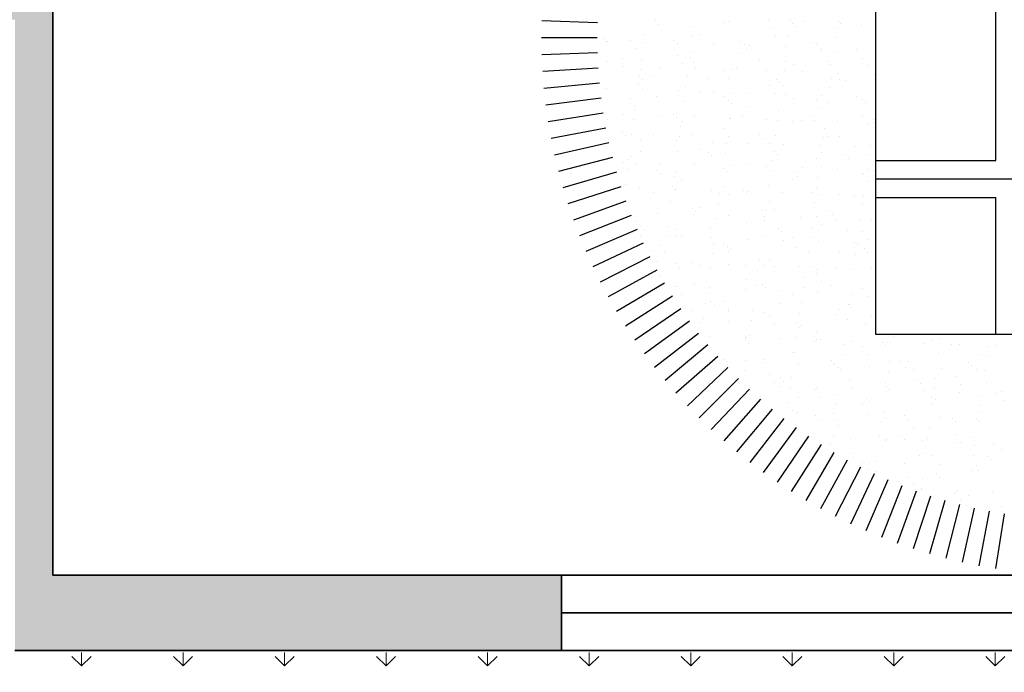
# Model space of a CAD drawing. Units: inches. Extents: x 1566 to 2546, y 1087 to 2705.
# Tile 3 of 27: x 1820 to 1925, y 1201 to 1270. Entities that reach past the tile are written whole.
import ezdxf

# ---------------------------------------------------------------- set-up
doc = ezdxf.new("R2010")
doc.units = ezdxf.units.IN
for name, color, linetype, lineweight in [('A-FLOR-PATT', 3, 'Continuous', 13), ('A-FURN', 8, 'Continuous', 18), ('A-WALL', 7, 'Continuous', 35), ('A-WALL-PATT', 8, 'Continuous', 13)]:
    doc.layers.add(name, color=color, linetype=linetype, lineweight=lineweight)
for name, color, linetype in [('A-FRN', 11, 'Continuous'), ('A-HT', 15, 'Continuous'), ('L-HT', 1, 'Continuous')]:
    doc.layers.add(name, color=color, linetype=linetype)

# ---------------------------------------------------------------- blocks, each defined once
blk = doc.blocks.new('*X21')
at = {"color": 0}
for p, q in [((2.0018, 2.8313), (2.0018, 2.8313)), ((2.0087, 2.8252), (2.0087, 2.8252)), ((2.011, 2.8229), (2.011, 2.8229)), ((2.0652, 2.8233), (2.0652, 2.8233)), ((2.1366, 2.8246), (2.1366, 2.8246)), ((2.2048, 2.8269), (2.2048, 2.8269)), ((2.2209, 2.8236), (2.2209, 2.8236)), ((2.0545, 2.783), (2.0545, 2.783)), ((2.0763, 2.7783), (2.0763, 2.7783)), ((2.2072, 2.78), (2.2072, 2.78)), ((2.2546, 2.7813), (2.2546, 2.7813)), ((2.2638, 2.7728), (2.2638, 2.7728)), ((2.32, 2.7605), (2.32, 2.7605)), ((2.3282, 2.7662), (2.3282, 2.7662)), ((2.3351, 2.7793), (2.3351, 2.7793)), ((2.3542, 2.7696), (2.3542, 2.7696)), ((2.3949, 2.775), (2.3949, 2.775)), ((2.0085, 2.7599), (2.0085, 2.7599)), ((2.0296, 2.7465), (2.0296, 2.7465)), ((2.0851, 2.7342), (2.0851, 2.7342)), ((2.1043, 2.7374), (2.1043, 2.7374)), ((2.1257, 2.7395), (2.1257, 2.7395)), ((2.1643, 2.7602), (2.1643, 2.7602)), ((2.1853, 2.7467), (2.1853, 2.7467)), ((2.1936, 2.7485), (2.1936, 2.7485)), ((2.2196, 2.7519), (2.2196, 2.7519)), ((2.2603, 2.7573), (2.2603, 2.7573)), ((2.341, 2.747), (2.341, 2.747)), ((2.4057, 2.7348), (2.4057, 2.7348)), ((2.4967, 2.7473), (2.4967, 2.7473)), ((2.5336, 2.7341), (2.5336, 2.7341)), ((1.9911, 2.7218), (1.9911, 2.7218)), ((2.0118, 2.7288), (2.0118, 2.7288)), ((2.059, 2.7308), (2.059, 2.7308)), ((2.1135, 2.729), (2.1135, 2.729)), ((2.1397, 2.7282), (2.1397, 2.7282)), ((2.2748, 2.7331), (2.2748, 2.7331)), ((2.3073, 2.733), (2.3073, 2.733)), ((2.5074, 2.7313), (2.5074, 2.7313)), ((2.5166, 2.7228), (2.5166, 2.7228)), ((1.954, 2.6935), (1.954, 2.6935)), ((1.9632, 2.6851), (1.9632, 2.6851)), ((2.0794, 2.682), (2.0794, 2.682)), ((2.1055, 2.6981), (2.1055, 2.6981)), ((2.157, 2.6891), (2.157, 2.6891)), ((2.2103, 2.6836), (2.2103, 2.6836)), ((2.2612, 2.6984), (2.2612, 2.6984)), ((2.3382, 2.683), (2.3382, 2.683)), ((2.3571, 2.6874), (2.3571, 2.6874)), ((2.4169, 2.6987), (2.4169, 2.6987)), ((2.4733, 2.6879), (2.4733, 2.6879)), ((2.5601, 2.683), (2.5601, 2.683)), ((2.5727, 2.6989), (2.5727, 2.6989)), ((2.6042, 2.6895), (2.6042, 2.6895)), ((2.3663, 2.6789), (2.3663, 2.6789)), ((2.5089, 2.6605), (2.5089, 2.6605)), ((2.5349, 2.664), (2.5349, 2.664)), ((2.5756, 2.6693), (2.5756, 2.6693)), ((2.6435, 2.6783), (2.6435, 2.6783)), ((2.0067, 2.6452), (2.0067, 2.6452)), ((2.015, 2.6325), (2.015, 2.6325)), ((2.0489, 2.6347), (2.0489, 2.6347)), ((2.1429, 2.6319), (2.1429, 2.6319)), ((2.2046, 2.635), (2.2046, 2.635)), ((2.2068, 2.6435), (2.2068, 2.6435)), ((2.216, 2.635), (2.216, 2.635)), ((2.2657, 2.6285), (2.2657, 2.6285)), ((2.2779, 2.6367), (2.2779, 2.6367)), ((2.3064, 2.6339), (2.3064, 2.6339)), ((2.3603, 2.6352), (2.3603, 2.6352)), ((2.3743, 2.6428), (2.3743, 2.6428)), ((2.4003, 2.6462), (2.4003, 2.6462)), ((2.4088, 2.6384), (2.4088, 2.6384)), ((2.4098, 2.6391), (2.4098, 2.6391)), ((2.441, 2.6516), (2.441, 2.6516)), ((2.516, 2.6355), (2.516, 2.6355)), ((2.5367, 2.6378), (2.5367, 2.6378)), ((2.6099, 2.6374), (2.6099, 2.6374)), ((2.6191, 2.6289), (2.6191, 2.6289)), ((2.6718, 2.6427), (2.6718, 2.6427)), ((2.6718, 2.6358), (2.6718, 2.6358)), ((2.07, 2.6213), (2.07, 2.6213)), ((2.1051, 2.6074), (2.1051, 2.6074)), ((2.1312, 2.6108), (2.1312, 2.6108)), ((2.1718, 2.6162), (2.1718, 2.6162)), ((2.2257, 2.6215), (2.2257, 2.6215)), ((2.2397, 2.6251), (2.2397, 2.6251)), ((2.3814, 2.6218), (2.3814, 2.6218)), ((2.5371, 2.6221), (2.5371, 2.6221)), ((2.6928, 2.6224), (2.6928, 2.6224)), ((1.9705, 2.5897), (1.9705, 2.5897)), ((1.9966, 2.5931), (1.9966, 2.5931)), ((2.0372, 2.5984), (2.0372, 2.5984)), ((2.0565, 2.5996), (2.0565, 2.5996)), ((2.0657, 2.5912), (2.0657, 2.5912)), ((2.0826, 2.5856), (2.0826, 2.5856)), ((2.2135, 2.5873), (2.2135, 2.5873)), ((2.2595, 2.5952), (2.2595, 2.5952)), ((2.3414, 2.5867), (2.3414, 2.5867)), ((2.4595, 2.5935), (2.4595, 2.5935)), ((2.4688, 2.585), (2.4688, 2.585)), ((2.4764, 2.5915), (2.4764, 2.5915)), ((2.6073, 2.5932), (2.6073, 2.5932)), ((2.6626, 2.589), (2.6626, 2.589)), ((2.7352, 2.5926), (2.7352, 2.5926)), ((1.9902, 2.5726), (1.9902, 2.5726)), ((2.1092, 2.5513), (2.1092, 2.5513)), ((2.1459, 2.5729), (2.1459, 2.5729)), ((2.3016, 2.5732), (2.3016, 2.5732)), ((2.3092, 2.5496), (2.3092, 2.5496)), ((2.4573, 2.5735), (2.4573, 2.5735)), ((2.613, 2.5737), (2.613, 2.5737)), ((2.6896, 2.5549), (2.6896, 2.5549)), ((2.7156, 2.5583), (2.7156, 2.5583)), ((2.7563, 2.5636), (2.7563, 2.5636)), ((2.7687, 2.574), (2.7687, 2.574)), ((2.0181, 2.5361), (2.0181, 2.5361)), ((2.146, 2.5355), (2.146, 2.5355)), ((2.2811, 2.5404), (2.2811, 2.5404)), ((2.3185, 2.5411), (2.3185, 2.5411)), ((2.412, 2.5421), (2.412, 2.5421)), ((2.4464, 2.5229), (2.4464, 2.5229)), ((2.4871, 2.5282), (2.4871, 2.5282)), ((2.5123, 2.5452), (2.5123, 2.5452)), ((2.5399, 2.5415), (2.5399, 2.5415)), ((2.555, 2.5371), (2.555, 2.5371)), ((2.581, 2.5406), (2.581, 2.5406)), ((2.6217, 2.5459), (2.6217, 2.5459)), ((2.6749, 2.5463), (2.6749, 2.5463)), ((2.7123, 2.5434), (2.7123, 2.5434)), ((2.7216, 2.535), (2.7216, 2.535)), ((2.8058, 2.548), (2.8058, 2.548)), ((1.9547, 2.4958), (1.9547, 2.4958)), ((1.9589, 2.5074), (1.9589, 2.5074)), ((2.0893, 2.5095), (2.0893, 2.5095)), ((2.1104, 2.496), (2.1104, 2.496)), ((2.1589, 2.5057), (2.1589, 2.5057)), ((2.1682, 2.4973), (2.1682, 2.4973)), ((2.245, 2.5098), (2.245, 2.5098)), ((2.2661, 2.4963), (2.2661, 2.4963)), ((2.2858, 2.5017), (2.2858, 2.5017)), ((2.3118, 2.5051), (2.3118, 2.5051)), ((2.3525, 2.5105), (2.3525, 2.5105)), ((2.362, 2.5013), (2.362, 2.5013)), ((2.4007, 2.51), (2.4007, 2.51)), ((2.4204, 2.5194), (2.4204, 2.5194)), ((2.4218, 2.4966), (2.4218, 2.4966)), ((2.4796, 2.4952), (2.4796, 2.4952)), ((2.5564, 2.5103), (2.5564, 2.5103)), ((2.562, 2.4996), (2.562, 2.4996)), ((2.5775, 2.4969), (2.5775, 2.4969)), ((2.6104, 2.4969), (2.6104, 2.4969)), ((2.7121, 2.5106), (2.7121, 2.5106)), ((2.7332, 2.4972), (2.7332, 2.4972)), ((2.7384, 2.4962), (2.7384, 2.4962)), ((2.7651, 2.4951), (2.7651, 2.4951)), ((2.8678, 2.5109), (2.8678, 2.5109)), ((2.8734, 2.5011), (2.8734, 2.5011)), ((2.8889, 2.4975), (2.8889, 2.4975)), ((2.0427, 2.4697), (2.0427, 2.4697)), ((2.0833, 2.4751), (2.0833, 2.4751)), ((2.0857, 2.4893), (2.0857, 2.4893)), ((2.1512, 2.484), (2.1512, 2.484)), ((2.1773, 2.4874), (2.1773, 2.4874)), ((2.2166, 2.4909), (2.2166, 2.4909)), ((2.2179, 2.4928), (2.2179, 2.4928)), ((2.3445, 2.4903), (2.3445, 2.4903)), ((2.5712, 2.4911), (2.5712, 2.4911)), ((2.0086, 2.4618), (2.0086, 2.4618)), ((2.0166, 2.4663), (2.0166, 2.4663)), ((2.0178, 2.4534), (2.0178, 2.4534)), ((2.0306, 2.4474), (2.0306, 2.4474)), ((2.1863, 2.4477), (2.1863, 2.4477)), ((2.2117, 2.4574), (2.2117, 2.4574)), ((2.2842, 2.4441), (2.2842, 2.4441)), ((2.342, 2.448), (2.342, 2.448)), ((2.4117, 2.4557), (2.4117, 2.4557)), ((2.4151, 2.4457), (2.4151, 2.4457)), ((2.4209, 2.4472), (2.4209, 2.4472)), ((2.4977, 2.4483), (2.4977, 2.4483)), ((2.543, 2.4451), (2.543, 2.4451)), ((2.6147, 2.4513), (2.6147, 2.4513)), ((2.6534, 2.4485), (2.6534, 2.4485)), ((2.6781, 2.45), (2.6781, 2.45)), ((2.8089, 2.4516), (2.8089, 2.4516)), ((2.8091, 2.4488), (2.8091, 2.4488)), ((2.8148, 2.4495), (2.8148, 2.4495)), ((2.8703, 2.4492), (2.8703, 2.4492)), ((2.8963, 2.4526), (2.8963, 2.4526)), ((2.9368, 2.451), (2.9368, 2.451)), ((2.0213, 2.4398), (2.0213, 2.4398)), ((2.1492, 2.4392), (2.1492, 2.4392)), ((2.6271, 2.4172), (2.6271, 2.4172)), ((2.6678, 2.4225), (2.6678, 2.4225)), ((2.7357, 2.4315), (2.7357, 2.4315)), ((2.7617, 2.4349), (2.7617, 2.4349)), ((2.8024, 2.4403), (2.8024, 2.4403)), ((2.824, 2.4411), (2.824, 2.4411)), ((2.0613, 2.4135), (2.0613, 2.4135)), ((2.0889, 2.3929), (2.0889, 2.3929)), ((2.2198, 2.3946), (2.2198, 2.3946)), ((2.2614, 2.4118), (2.2614, 2.4118)), ((2.2706, 2.4033), (2.2706, 2.4033)), ((2.3477, 2.394), (2.3477, 2.394)), ((2.4644, 2.4074), (2.4644, 2.4074)), ((2.4665, 2.396), (2.4665, 2.396)), ((2.4827, 2.3988), (2.4827, 2.3988)), ((2.4925, 2.3995), (2.4925, 2.3995)), ((2.5332, 2.4048), (2.5332, 2.4048)), ((2.6011, 2.4138), (2.6011, 2.4138)), ((2.6136, 2.4005), (2.6136, 2.4005)), ((2.6645, 2.4057), (2.6645, 2.4057)), ((2.6737, 2.3972), (2.6737, 2.3972)), ((2.7415, 2.3999), (2.7415, 2.3999)), ((2.8675, 2.4012), (2.8675, 2.4012)), ((2.8765, 2.4048), (2.8765, 2.4048)), ((1.9538, 2.3881), (1.9538, 2.3881)), ((1.974, 2.384), (1.974, 2.384)), ((1.9951, 2.3706), (1.9951, 2.3706)), ((2.1111, 2.3679), (2.1111, 2.3679)), ((2.1297, 2.3843), (2.1297, 2.3843)), ((2.1508, 2.3708), (2.1508, 2.3708)), ((2.2234, 2.364), (2.2234, 2.364)), ((2.264, 2.3694), (2.264, 2.3694)), ((2.2854, 2.3846), (2.2854, 2.3846)), ((2.3065, 2.3711), (2.3065, 2.3711)), ((2.3141, 2.3635), (2.3141, 2.3635)), ((2.3319, 2.3783), (2.3319, 2.3783)), ((2.3579, 2.3817), (2.3579, 2.3817)), ((2.3986, 2.3871), (2.3986, 2.3871)), ((2.4411, 2.3848), (2.4411, 2.3848)), ((2.4622, 2.3714), (2.4622, 2.3714)), ((2.5968, 2.3851), (2.5968, 2.3851)), ((2.6179, 2.3717), (2.6179, 2.3717)), ((2.7525, 2.3854), (2.7525, 2.3854)), ((2.7736, 2.372), (2.7736, 2.372)), ((2.9082, 2.3857), (2.9082, 2.3857)), ((2.9293, 2.3723), (2.9293, 2.3723)), ((2.0244, 2.3435), (2.0244, 2.3435)), ((2.0627, 2.3429), (2.0627, 2.3429)), ((2.0888, 2.3463), (2.0888, 2.3463)), ((2.1203, 2.3595), (2.1203, 2.3595)), ((2.1294, 2.3517), (2.1294, 2.3517)), ((2.1523, 2.3429), (2.1523, 2.3429)), ((2.1973, 2.3606), (2.1973, 2.3606)), ((2.2874, 2.3477), (2.2874, 2.3477)), ((2.4183, 2.3494), (2.4183, 2.3494)), ((2.5142, 2.3618), (2.5142, 2.3618)), ((2.5234, 2.3533), (2.5234, 2.3533)), ((2.5462, 2.3488), (2.5462, 2.3488)), ((2.6812, 2.3536), (2.6812, 2.3536)), ((2.7172, 2.3573), (2.7172, 2.3573)), ((2.8121, 2.3553), (2.8121, 2.3553)), ((2.9173, 2.3556), (2.9173, 2.3556)), ((2.9265, 2.3472), (2.9265, 2.3472)), ((2.94, 2.3547), (2.94, 2.3547)), ((1.9542, 2.3286), (1.9542, 2.3286)), ((1.9608, 2.324), (1.9608, 2.324)), ((1.97, 2.3156), (1.97, 2.3156)), ((1.9948, 2.3339), (1.9948, 2.3339)), ((2.071, 2.3222), (2.071, 2.3222)), ((2.1638, 2.3196), (2.1638, 2.3196)), ((2.2267, 2.3225), (2.2267, 2.3225)), ((2.3639, 2.3179), (2.3639, 2.3179)), ((2.3731, 2.3094), (2.3731, 2.3094)), ((2.3824, 2.3228), (2.3824, 2.3228)), ((2.5381, 2.323), (2.5381, 2.323)), ((2.5669, 2.3135), (2.5669, 2.3135)), ((2.6938, 2.3233), (2.6938, 2.3233)), ((2.767, 2.3117), (2.767, 2.3117)), ((2.8078, 2.3115), (2.8078, 2.3115)), ((2.8485, 2.3169), (2.8485, 2.3169)), ((2.8495, 2.3236), (2.8495, 2.3236)), ((2.9164, 2.3258), (2.9164, 2.3258)), ((2.9424, 2.3292), (2.9424, 2.3292)), ((2.983, 2.3346), (2.983, 2.3346)), ((3.0052, 2.3239), (3.0052, 2.3239)), ((3.0106, 2.3101), (3.0106, 2.3101)), ((1.957, 2.2917), (1.957, 2.2917)), ((2.092, 2.2966), (2.092, 2.2966)), ((2.2229, 2.2983), (2.2229, 2.2983)), ((2.3508, 2.2976), (2.3508, 2.2976)), ((2.4859, 2.3025), (2.4859, 2.3025)), ((2.6167, 2.3042), (2.6167, 2.3042)), ((2.6472, 2.2904), (2.6472, 2.2904)), ((2.6732, 2.2938), (2.6732, 2.2938)), ((2.7139, 2.2992), (2.7139, 2.2992)), ((2.7447, 2.3036), (2.7447, 2.3036)), ((2.7762, 2.3033), (2.7762, 2.3033)), ((2.7818, 2.3081), (2.7818, 2.3081)), ((2.8797, 2.3084), (2.8797, 2.3084)), ((2.97, 2.3073), (2.97, 2.3073)), ((2.0135, 2.2757), (2.0135, 2.2757)), ((2.0144, 2.2588), (2.0144, 2.2588)), ((2.1701, 2.2591), (2.1701, 2.2591)), ((2.2136, 2.274), (2.2136, 2.274)), ((2.2228, 2.2656), (2.2228, 2.2656)), ((2.3258, 2.2594), (2.3258, 2.2594)), ((2.404, 2.2584), (2.404, 2.2584)), ((2.4166, 2.2696), (2.4166, 2.2696)), ((2.4447, 2.2637), (2.4447, 2.2637)), ((2.4815, 2.2596), (2.4815, 2.2596)), ((2.5126, 2.2727), (2.5126, 2.2727)), ((2.5386, 2.2761), (2.5386, 2.2761)), ((2.5793, 2.2814), (2.5793, 2.2814)), ((2.6167, 2.2679), (2.6167, 2.2679)), ((2.6259, 2.2594), (2.6259, 2.2594)), ((2.6372, 2.2599), (2.6372, 2.2599)), ((2.6844, 2.2573), (2.6844, 2.2573)), ((2.7929, 2.2602), (2.7929, 2.2602)), ((2.8152, 2.259), (2.8152, 2.259)), ((2.8197, 2.2634), (2.8197, 2.2634)), ((2.9431, 2.2584), (2.9431, 2.2584)), ((2.9486, 2.2605), (2.9486, 2.2605)), ((3.0198, 2.2617), (3.0198, 2.2617)), ((3.0782, 2.2632), (3.0782, 2.2632)), ((2.0276, 2.2471), (2.0276, 2.2471)), ((2.0354, 2.2454), (2.0354, 2.2454)), ((2.0633, 2.2301), (2.0633, 2.2301)), ((2.1555, 2.2465), (2.1555, 2.2465)), ((2.1912, 2.2456), (2.1912, 2.2456)), ((2.2434, 2.2372), (2.2434, 2.2372)), ((2.2695, 2.2406), (2.2695, 2.2406)), ((2.2905, 2.2514), (2.2905, 2.2514)), ((2.3101, 2.246), (2.3101, 2.246)), ((2.3469, 2.2459), (2.3469, 2.2459)), ((2.378, 2.2549), (2.378, 2.2549)), ((2.4214, 2.253), (2.4214, 2.253)), ((2.5026, 2.2462), (2.5026, 2.2462)), ((2.5493, 2.2524), (2.5493, 2.2524)), ((2.6583, 2.2465), (2.6583, 2.2465)), ((2.814, 2.2468), (2.814, 2.2468)), ((2.9697, 2.2471), (2.9697, 2.2471)), ((3.029, 2.2533), (3.029, 2.2533)), ((2.0003, 2.2052), (2.0003, 2.2052)), ((2.0409, 2.2106), (2.0409, 2.2106)), ((2.0725, 2.2217), (2.0725, 2.2217)), ((2.1088, 2.2195), (2.1088, 2.2195)), ((2.1349, 2.2229), (2.1349, 2.2229)), ((2.1755, 2.2283), (2.1755, 2.2283)), ((2.2663, 2.2257), (2.2663, 2.2257)), ((2.4664, 2.224), (2.4664, 2.224)), ((2.4756, 2.2155), (2.4756, 2.2155)), ((2.489, 2.2062), (2.489, 2.2062)), ((2.6199, 2.2078), (2.6199, 2.2078)), ((2.6694, 2.2196), (2.6694, 2.2196)), ((2.7478, 2.2072), (2.7478, 2.2072)), ((2.8695, 2.2178), (2.8695, 2.2178)), ((2.8787, 2.2094), (2.8787, 2.2094)), ((2.8828, 2.2121), (2.8828, 2.2121)), ((2.9885, 2.2058), (2.9885, 2.2058)), ((3.0137, 2.2138), (3.0137, 2.2138)), ((3.0291, 2.2112), (3.0291, 2.2112)), ((3.0725, 2.2134), (3.0725, 2.2134)), ((3.0971, 2.2201), (3.0971, 2.2201)), ((1.9556, 2.1967), (1.9556, 2.1967)), ((1.9601, 2.1954), (1.9601, 2.1954)), ((1.9743, 2.2018), (1.9743, 2.2018)), ((2.0952, 2.2002), (2.0952, 2.2002)), ((2.1114, 2.197), (2.1114, 2.197)), ((2.116, 2.1818), (2.116, 2.1818)), ((2.2261, 2.2019), (2.2261, 2.2019)), ((2.2671, 2.1973), (2.2671, 2.1973)), ((2.3161, 2.1801), (2.3161, 2.1801)), ((2.354, 2.2013), (2.354, 2.2013)), ((2.4228, 2.1976), (2.4228, 2.1976)), ((2.5785, 2.1978), (2.5785, 2.1978)), ((2.7342, 2.1981), (2.7342, 2.1981)), ((2.8279, 2.1847), (2.8279, 2.1847)), ((2.8539, 2.1881), (2.8539, 2.1881)), ((2.8899, 2.1984), (2.8899, 2.1984)), ((2.8946, 2.1935), (2.8946, 2.1935)), ((2.9625, 2.2024), (2.9625, 2.2024)), ((3.0456, 2.1987), (3.0456, 2.1987)), ((2.0307, 2.1508), (2.0307, 2.1508)), ((2.1586, 2.1502), (2.1586, 2.1502)), ((2.2937, 2.155), (2.2937, 2.155)), ((2.3253, 2.1717), (2.3253, 2.1717)), ((2.4246, 2.1567), (2.4246, 2.1567)), ((2.5191, 2.1757), (2.5191, 2.1757)), ((2.5525, 2.1561), (2.5525, 2.1561)), ((2.5847, 2.1527), (2.5847, 2.1527)), ((2.6254, 2.158), (2.6254, 2.158)), ((2.6875, 2.161), (2.6875, 2.161)), ((2.6933, 2.167), (2.6933, 2.167)), ((2.7192, 2.174), (2.7192, 2.174)), ((2.7193, 2.1704), (2.7193, 2.1704)), ((2.7284, 2.1655), (2.7284, 2.1655)), ((2.76, 2.1758), (2.76, 2.1758)), ((2.8184, 2.1626), (2.8184, 2.1626)), ((2.9222, 2.1695), (2.9222, 2.1695)), ((2.9463, 2.162), (2.9463, 2.162)), ((3.0813, 2.1669), (3.0813, 2.1669)), ((3.1223, 2.1678), (3.1223, 2.1678)), ((3.1315, 2.1594), (3.1315, 2.1594)), ((1.9657, 2.1379), (1.9657, 2.1379)), ((2.0547, 2.1336), (2.0547, 2.1336)), ((2.1658, 2.1362), (2.1658, 2.1362)), ((2.175, 2.1278), (2.175, 2.1278)), ((2.2105, 2.1339), (2.2105, 2.1339)), ((2.3662, 2.1341), (2.3662, 2.1341)), ((2.3688, 2.1318), (2.3688, 2.1318)), ((2.4241, 2.1315), (2.4241, 2.1315)), ((2.4501, 2.135), (2.4501, 2.135)), ((2.4908, 2.1403), (2.4908, 2.1403)), ((2.5219, 2.1344), (2.5219, 2.1344)), ((2.5587, 2.1493), (2.5587, 2.1493)), ((2.5689, 2.1301), (2.5689, 2.1301)), ((2.6776, 2.1347), (2.6776, 2.1347)), ((2.7719, 2.1257), (2.7719, 2.1257)), ((2.8333, 2.135), (2.8333, 2.135)), ((2.972, 2.1239), (2.972, 2.1239)), ((2.989, 2.1353), (2.989, 2.1353)), ((3.1447, 2.1356), (3.1447, 2.1356)), ((2.0758, 2.1201), (2.0758, 2.1201)), ((2.0983, 2.1039), (2.0983, 2.1039)), ((2.2216, 2.1049), (2.2216, 2.1049)), ((2.2292, 2.1056), (2.2292, 2.1056)), ((2.2315, 2.1204), (2.2315, 2.1204)), ((2.2895, 2.1138), (2.2895, 2.1138)), ((2.3156, 2.1173), (2.3156, 2.1173)), ((2.3562, 2.1226), (2.3562, 2.1226)), ((2.3571, 2.105), (2.3571, 2.105)), ((2.3872, 2.1207), (2.3872, 2.1207)), ((2.4922, 2.1098), (2.4922, 2.1098)), ((2.5429, 2.121), (2.5429, 2.121)), ((2.5781, 2.1216), (2.5781, 2.1216)), ((2.623, 2.1115), (2.623, 2.1115)), ((2.6987, 2.1213), (2.6987, 2.1213)), ((2.751, 2.1109), (2.751, 2.1109)), ((2.8544, 2.1216), (2.8544, 2.1216)), ((2.886, 2.1157), (2.886, 2.1157)), ((2.9812, 2.1155), (2.9812, 2.1155)), ((3.0101, 2.1218), (3.0101, 2.1218)), ((3.0169, 2.1174), (3.0169, 2.1174)), ((3.1448, 2.1168), (3.1448, 2.1168)), ((3.1658, 2.1221), (3.1658, 2.1221)), ((3.1692, 2.1002), (3.1692, 2.1002)), ((2.8216, 2.08), (2.8216, 2.08)), ((2.8309, 2.0716), (2.8309, 2.0716)), ((2.9303, 2.0732), (2.9303, 2.0732)), ((3.0086, 2.079), (3.0086, 2.079)), ((3.0247, 2.0756), (3.0247, 2.0756)), ((3.0346, 2.0825), (3.0346, 2.0825)), ((3.0752, 2.0878), (3.0752, 2.0878)), ((3.0845, 2.0705), (3.0845, 2.0705)), ((3.086, 2.0735), (3.086, 2.0735)), ((3.1432, 2.0968), (3.1432, 2.0968)), ((2.8061, 2.0524), (2.8061, 2.0524)), ((2.8215, 2.0663), (2.8215, 2.0663)), ((2.874, 2.0613), (2.874, 2.0613)), ((2.9, 2.0647), (2.9, 2.0647)), ((2.9407, 2.0701), (2.9407, 2.0701)), ((2.9494, 2.0657), (2.9494, 2.0657)), ((2.8744, 2.0317), (2.8744, 2.0317)), ((2.8891, 2.0194), (2.8891, 2.0194)), ((3.02, 2.0211), (3.02, 2.0211)), ((3.0744, 2.03), (3.0744, 2.03)), ((3.0837, 2.0216), (3.0837, 2.0216)), ((3.1479, 2.0205), (3.1479, 2.0205)), ((2.8737, 2.0098), (2.8737, 2.0098)), ((2.8947, 1.9964), (2.8947, 1.9964)), ((3.0294, 2.0101), (3.0294, 2.0101)), ((3.0505, 1.9966), (3.0505, 1.9966)), ((3.1851, 2.0104), (3.1851, 2.0104)), ((3.2062, 1.9969), (3.2062, 1.9969)), ((2.8247, 1.9699), (2.8247, 1.9699)), ((2.9241, 1.9861), (2.9241, 1.9861)), ((2.9333, 1.9777), (2.9333, 1.9777)), ((2.9526, 1.9693), (2.9526, 1.9693)), ((3.0876, 1.9742), (3.0876, 1.9742)), ((3.1213, 1.9644), (3.1213, 1.9644)), ((3.1272, 1.9817), (3.1272, 1.9817)), ((3.1893, 1.9734), (3.1893, 1.9734)), ((3.2153, 1.9768), (3.2153, 1.9768)), ((3.2185, 1.9759), (3.2185, 1.9759)), ((2.8149, 1.9477), (2.8149, 1.9477)), ((2.9201, 1.9379), (2.9201, 1.9379)), ((2.9461, 1.9414), (2.9461, 1.9414)), ((2.9707, 1.948), (2.9707, 1.948)), ((2.9768, 1.9378), (2.9768, 1.9378)), ((2.9868, 1.9467), (2.9868, 1.9467)), ((3.0547, 1.9556), (3.0547, 1.9556)), ((3.0807, 1.9591), (3.0807, 1.9591)), ((3.1264, 1.9483), (3.1264, 1.9483)), ((2.8115, 1.9236), (2.8115, 1.9236)), ((2.8522, 1.929), (2.8522, 1.929)), ((2.8923, 1.9231), (2.8923, 1.9231)), ((3.0232, 1.9247), (3.0232, 1.9247)), ((3.1511, 1.9241), (3.1511, 1.9241)), ((3.1769, 1.9361), (3.1769, 1.9361)), ((3.1861, 1.9277), (3.1861, 1.9277)), ((2.8265, 1.894), (2.8265, 1.894)), ((2.914, 1.8846), (2.914, 1.8846)), ((3.0266, 1.8922), (3.0266, 1.8922)), ((3.0697, 1.8849), (3.0697, 1.8849)), ((3.2255, 1.8852), (3.2255, 1.8852)), ((3.2296, 1.8878), (3.2296, 1.8878)), ((2.8278, 1.8736), (2.8278, 1.8736)), ((2.9351, 1.8712), (2.9351, 1.8712)), ((2.9557, 1.873), (2.9557, 1.873)), ((3.0358, 1.8838), (3.0358, 1.8838)), ((3.0908, 1.8779), (3.0908, 1.8779)), ((3.0908, 1.8714), (3.0908, 1.8714)), ((3.2217, 1.8795), (3.2217, 1.8795)), ((3.2465, 1.8717), (3.2465, 1.8717)), ((2.8763, 1.8484), (2.8763, 1.8484)), ((2.8855, 1.8399), (2.8855, 1.8399)), ((3.0793, 1.8439), (3.0793, 1.8439)), ((3.1008, 1.8323), (3.1008, 1.8323)), ((3.1268, 1.8357), (3.1268, 1.8357)), ((3.1674, 1.841), (3.1674, 1.841)), ((3.2354, 1.85), (3.2354, 1.85)), ((3.2614, 1.8534), (3.2614, 1.8534)), ((2.8553, 1.8225), (2.8553, 1.8225)), ((2.8954, 1.8267), (2.8954, 1.8267)), ((2.8983, 1.8056), (2.8983, 1.8056)), ((2.9662, 1.8145), (2.9662, 1.8145)), ((2.9922, 1.818), (2.9922, 1.818)), ((3.011, 1.8228), (3.011, 1.8228)), ((3.0263, 1.8284), (3.0263, 1.8284)), ((3.0329, 1.8233), (3.0329, 1.8233)), ((3.1542, 1.8278), (3.1542, 1.8278)), ((3.1667, 1.8231), (3.1667, 1.8231)), ((2.8316, 1.7968), (2.8316, 1.7968)), ((2.8576, 1.8002), (2.8576, 1.8002)), ((2.929, 1.8), (2.929, 1.8)), ((3.0939, 1.7815), (3.0939, 1.7815)), ((3.1291, 1.7983), (3.1291, 1.7983)), ((3.1383, 1.7899), (3.1383, 1.7899)), ((3.2248, 1.7832), (3.2248, 1.7832)), ((2.831, 1.7773), (2.831, 1.7773)), ((2.9544, 1.7594), (2.9544, 1.7594)), ((2.9589, 1.7766), (2.9589, 1.7766)), ((2.9788, 1.7544), (2.9788, 1.7544)), ((3.1101, 1.7597), (3.1101, 1.7597)), ((3.2658, 1.7599), (3.2658, 1.7599))]:
    blk.add_line(p, q, dxfattribs=at)
blk = doc.blocks.new('A$C6796526C')
at = {"layer": 'A-FRN'}
blk.add_lwpolyline([(0.65, 2.8), (0.65, 0.9), (2.25, 0.9), (2.25, 2.8)], dxfattribs=at)
at = {"layer": 'A-HT'}
for p, q in [((2.734, 1.2466), (2.8821, 1.2232)), ((2.727, 1.2064), (2.8743, 1.1783)), ((2.7187, 1.1664), (2.8651, 1.1337)), ((2.7092, 1.1267), (2.8544, 1.0894)), ((2.6984, 1.0873), (2.8424, 1.0455)), ((2.6864, 1.0483), (2.829, 1.0019)), ((2.6731, 1.0096), (2.8143, 0.9588)), ((2.6587, 0.9714), (2.7982, 0.9162)), ((2.6431, 0.9337), (2.7807, 0.8741)), ((2.6263, 0.8965), (2.762, 0.8326)), ((2.6083, 0.8598), (2.742, 0.7917)), ((2.5892, 0.8237), (2.7206, 0.7515)), ((2.569, 0.7882), (2.6981, 0.7119)), ((2.5476, 0.7534), (2.6743, 0.6731)), ((2.5252, 0.7193), (2.6493, 0.635)), ((2.5017, 0.6859), (2.6231, 0.5977)), ((2.4772, 0.6532), (2.5957, 0.5613)), ((2.4517, 0.6213), (2.5672, 0.5257)), ((2.4251, 0.5903), (2.5377, 0.4911)), ((2.3977, 0.5601), (2.507, 0.4574)), ((2.3692, 0.5308), (2.4753, 0.4247)), ((2.3399, 0.5023), (2.4426, 0.393)), ((2.3097, 0.4749), (2.4089, 0.3623)), ((2.2787, 0.4483), (2.3743, 0.3328)), ((2.2148, 0.3985), (2.303, 0.2772)), ((2.2474, 0.423), (2.3394, 0.3045)), ((2.1814, 0.375), (2.2657, 0.251)), ((2.1472, 0.3526), (2.2276, 0.226)), ((2.1124, 0.3313), (2.1888, 0.2022)), ((2.0769, 0.311), (2.1492, 0.1796)), ((2.0042, 0.274), (2.068, 0.1382)), ((2.0409, 0.2919), (2.109, 0.1583)), ((1.9292, 0.2415), (1.9844, 0.1021)), ((1.967, 0.2572), (2.0265, 0.1195)), ((1.8517, 0.2136), (1.8981, 0.071)), ((1.891, 0.2271), (1.9418, 0.086)), ((1.7733, 0.1908), (1.8106, 0.0456)), ((1.8127, 0.2016), (1.8545, 0.0576)), ((1.6129, 0.1603), (1.6317, 0.0114)), ((1.6534, 0.166), (1.6768, 0.0179)), ((1.6936, 0.173), (1.7217, 0.0257)), ((1.7336, 0.1813), (1.7663, 0.0349)), ((1.4092, 0.1506), (1.4045, 0.0007)), ((1.45, 0.15), (1.45, 0)), ((1.4908, 0.1506), (1.4955, 0.0007)), ((1.5316, 0.1526), (1.541, 0.0029)), ((1.5723, 0.1558), (1.5865, 0.0064))]:
    blk.add_line(p, q, dxfattribs=at)
at = {"layer": 'L-HT'}
for p, q in [((1.8309, 0.9), (1.8309, 2.2094)), ((1.7809, 1.2249), (0.65, 1.2249)), ((1.7809, 0.9), (1.7809, 1.2249)), ((1.8809, 0.9), (1.8809, 1.2249)), ((2.25, 1.2249), (1.8809, 1.2249))]:
    blk.add_line(p, q, dxfattribs=at)
at = {"layer": 'A-HT', "extrusion": (0, 0, -1), "zscale": -1, "rotation": 180}
blk.add_blockref('*X21', (0.55, 3), dxfattribs=at)

msp = doc.modelspace()

# ---------------------------------------------------------------- hatches: boundary and pattern name
at = {"layer": 'A-FLOR-PATT'}
h = msp.add_hatch(dxfattribs=at)
h.set_pattern_fill('GRASS', color=256, scale=0.3)
h.paths.add_polyline_path([(1745.53, 1270.2), (1645.53, 1270.2), (1645.53, 1159.2), (1745.53, 1159.2)])
h.paths.add_polyline_path([(1993.53, 1203.2), (1819.53, 1203.2), (1819.53, 1155.2), (1993.53, 1155.2)])
h.paths.add_polyline_path([(1667.62, 1196.42), (1716.72, 1196.42), (1716.72, 1222.54), (1667.62, 1222.54)], flags=24)
h.paths.add_polyline_path([(1881.06, 1171.45), (1935.47, 1171.45), (1935.47, 1197.57), (1881.06, 1197.57)], flags=24)
at = {"layer": 'A-WALL-PATT'}
h = msp.add_hatch(color=256, dxfattribs=at)
h.dxf.hatch_style = 1
h.paths.add_polyline_path([(2001.53, 1778.2), (1641.53, 1778.2), (1641.53, 1746.2), (1649.53, 1746.2), (1649.53, 1770.2), (1769.53, 1770.2), (1769.53, 1650.2), (1767.53, 1650.2), (1767.53, 1648.2), (1767.53, 1646.2), (1819.53, 1646.2), (1819.53, 1650.2), (1773.53, 1650.2), (1773.53, 1770.2), (1941.53, 1770.2), (1941.53, 1756.2), (1945.53, 1756.2), (1945.53, 1770.2), (1993.53, 1770.2), (1993.53, 1650.2), (1945.53, 1650.2), (1945.53, 1652.2), (1943.53, 1652.2), (1941.53, 1652.2), (1941.53, 1650.2), (1867.53, 1650.2), (1867.53, 1642.2), (1871.53, 1642.2), (1871.53, 1646.2), (1993.53, 1646.2), (1993.53, 1526.2), (1871.53, 1526.2), (1871.53, 1606.2), (1867.53, 1606.2), (1867.53, 1522.2), (1993.53, 1522.2), (1993.53, 1387.2), (1959.53, 1387.2), (1959.53, 1397.2), (1955.53, 1397.2), (1955.53, 1387.2), (1903.53, 1387.2), (1903.53, 1383.2), (1993.53, 1383.2), (1993.53, 1364.3), (1993.53, 1211.2), (1939.53, 1211.2), (1939.53, 1203.2), (1993.53, 1203.2), (1993.53, 1154.2), (2001.53, 1154.2)])
h.paths.add_polyline_path([(1649.53, 1646.2), (1731.53, 1646.2), (1731.53, 1650.2), (1649.53, 1650.2), (1649.53, 1674.2), (1641.53, 1674.2), (1641.53, 1622.2), (1649.53, 1622.2)], flags=17)
h.paths.add_polyline_path([(1649.53, 1550.2), (1641.53, 1550.2), (1641.53, 1510.2), (1649.53, 1510.2), (1649.53, 1522.2), (1731.53, 1522.2), (1731.53, 1500.2), (1735.53, 1500.2), (1735.53, 1522.2), (1767.53, 1522.2), (1767.53, 1500.2), (1771.53, 1500.2), (1771.53, 1526.2), (1649.53, 1526.2)], flags=17)
h.paths.add_polyline_path([(1649.53, 1464.2), (1735.53, 1464.2), (1735.53, 1470.2), (1731.53, 1470.2), (1731.53, 1468.2), (1649.53, 1468.2), (1649.53, 1480.2), (1641.53, 1480.2), (1641.53, 1419.2), (1649.53, 1419.2)], flags=17)
h.paths.add_polyline_path([(1649.53, 1323.2), (1641.53, 1323.2), (1641.53, 1270.2), (1667.53, 1270.2), (1667.53, 1278.2), (1649.53, 1278.2)], flags=17)
h.paths.add_polyline_path([(1763.53, 1278.2), (1727.53, 1278.2), (1727.53, 1270.2), (1763.53, 1270.2)], flags=17)
h.paths.add_polyline_path([(1823.53, 1383.2), (1827.53, 1383.2), (1827.53, 1385.2), (1827.53, 1387.2), (1819.53, 1387.2), (1819.53, 1324.21), (1819.53, 1278.2), (1811.53, 1278.2), (1811.53, 1274.2), (1811.53, 1270.2), (1819.53, 1270.2), (1819.53, 1203.2), (1877.53, 1203.2), (1877.53, 1211.2), (1823.53, 1211.2)], flags=17)

# ---------------------------------------------------------------- linework, layer by layer
at = {"layer": 'A-WALL'}
for p, q in [((1823.53, 1211.2), (1823.53, 1383.2)), ((1823.53, 1211.2), (1993.53, 1211.2)), ((1877.53, 1211.2), (1877.53, 1203.2)), ((1877.53, 1211.2), (1877.53, 1203.2)), ((1877.53, 1207.2), (1939.53, 1207.2)), ((1877.53, 1207.2), (1939.53, 1207.2)), ((1819.53, 1203.2), (1993.53, 1203.2))]:
    msp.add_line(p, q, dxfattribs=at)

# ---------------------------------------------------------------- block references
at = {"layer": 'A-FURN', "xscale": 39.3701, "yscale": 39.3701, "zscale": 39.3701, "rotation": 270}
msp.add_blockref('A$C6796526C', (1875.42, 1325.37), dxfattribs=at)

doc.saveas('drawing.dxf')
